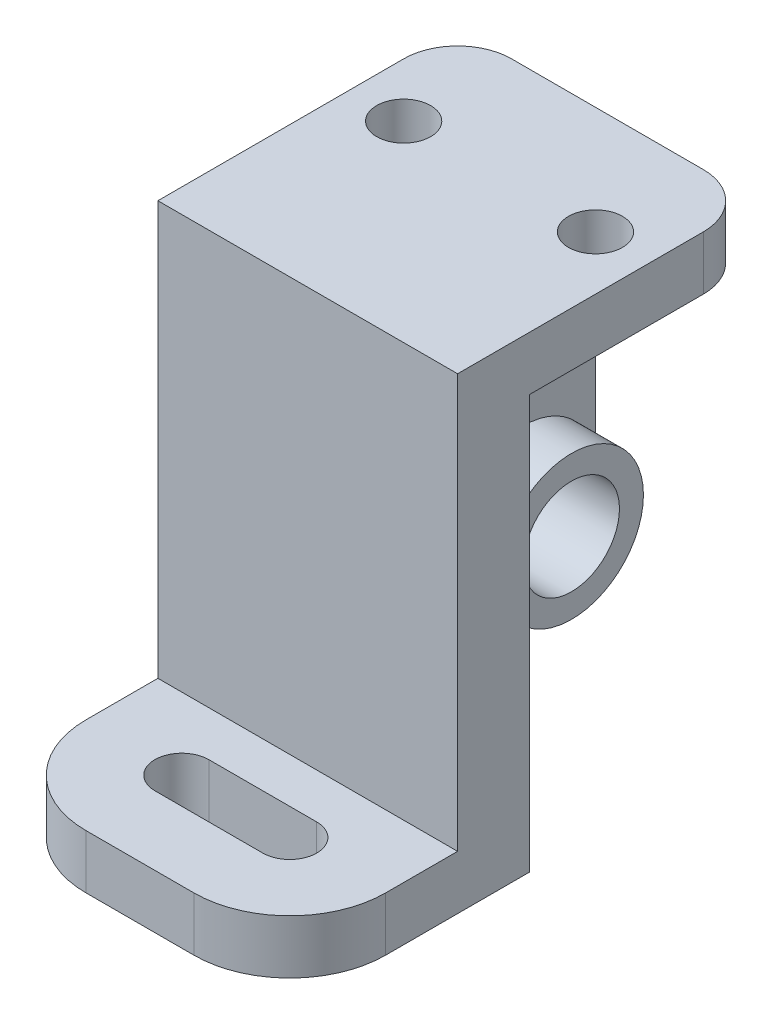
ISO-10303-21;
HEADER;
FILE_DESCRIPTION(('STEP AP214'),'2;1');
FILE_NAME('part.step','',(''),(''),'','','');
FILE_SCHEMA(('AUTOMOTIVE_DESIGN { 1 0 10303 214 1 1 1 1 }'));
ENDSEC;
DATA;
#1=APPLICATION_CONTEXT('core data for automotive mechanical design processes');
#2=APPLICATION_PROTOCOL_DEFINITION('international standard','automotive_design',2000,#1);
#3=PRODUCT_CONTEXT('',#1,'mechanical');
#4=PRODUCT('Part','Part','',(#3));
#5=PRODUCT_RELATED_PRODUCT_CATEGORY('part','',(#4));
#6=PRODUCT_DEFINITION_FORMATION('','',#4);
#7=PRODUCT_DEFINITION_CONTEXT('part definition',#1,'design');
#8=PRODUCT_DEFINITION('design','',#6,#7);
#9=PRODUCT_DEFINITION_SHAPE('','',#8);
#10=(LENGTH_UNIT() NAMED_UNIT(*) SI_UNIT(.MILLI.,.METRE.));
#11=(NAMED_UNIT(*) PLANE_ANGLE_UNIT() SI_UNIT($,.RADIAN.));
#12=(NAMED_UNIT(*) SI_UNIT($,.STERADIAN.) SOLID_ANGLE_UNIT());
#13=UNCERTAINTY_MEASURE_WITH_UNIT(LENGTH_MEASURE(1.E-05),#10,'distance_accuracy_value','');
#14=(GEOMETRIC_REPRESENTATION_CONTEXT(3) GLOBAL_UNCERTAINTY_ASSIGNED_CONTEXT((#13)) GLOBAL_UNIT_ASSIGNED_CONTEXT((#10,
#11,#12)) REPRESENTATION_CONTEXT('',''));
#15=CARTESIAN_POINT('',(0.,0.,0.));
#16=DIRECTION('',(0.,0.,1.));
#17=DIRECTION('',(1.,0.,0.));
#18=AXIS2_PLACEMENT_3D('',#15,#16,#17);
#19=CARTESIAN_POINT('',(-25.,9.,-20.));
#20=DIRECTION('',(0.,0.,1.));
#21=DIRECTION('',(1.,0.,0.));
#22=AXIS2_PLACEMENT_3D('',#19,#20,#21);
#23=PLANE('',#22);
#24=DIRECTION('',(0.,-1.,0.));
#25=VECTOR('',#24,1.);
#26=CARTESIAN_POINT('',(4.,0.,-20.));
#27=LINE('',#26,#25);
#28=CARTESIAN_POINT('',(4.,69.,-20.));
#29=VERTEX_POINT('',#28);
#30=CARTESIAN_POINT('',(4.,0.,-20.));
#31=VERTEX_POINT('',#30);
#32=EDGE_CURVE('E424',#29,#31,#27,.T.);
#33=ORIENTED_EDGE('',*,*,#32,.F.);
#34=DIRECTION('',(-1.,0.,0.));
#35=VECTOR('',#34,1.);
#36=CARTESIAN_POINT('',(0.,69.,-20.));
#37=LINE('',#36,#35);
#38=CARTESIAN_POINT('',(25.,69.,-20.));
#39=VERTEX_POINT('',#38);
#40=EDGE_CURVE('E66',#39,#29,#37,.T.);
#41=ORIENTED_EDGE('',*,*,#40,.F.);
#42=DIRECTION('',(0.,-1.,0.));
#43=VECTOR('',#42,1.);
#44=CARTESIAN_POINT('',(25.,9.,-20.));
#45=LINE('',#44,#43);
#46=CARTESIAN_POINT('',(25.,0.,-20.));
#47=VERTEX_POINT('',#46);
#48=EDGE_CURVE('E341',#39,#47,#45,.T.);
#49=ORIENTED_EDGE('',*,*,#48,.T.);
#50=DIRECTION('',(-1.,0.,0.));
#51=VECTOR('',#50,1.);
#52=CARTESIAN_POINT('',(-25.,0.,-20.));
#53=LINE('',#52,#51);
#54=EDGE_CURVE('E319',#47,#31,#53,.T.);
#55=ORIENTED_EDGE('',*,*,#54,.T.);
#56=EDGE_LOOP('',(#33,#41,#49,#55));
#57=FACE_BOUND('',#56,.T.);
#58=ADVANCED_FACE('F43',(#57),#23,.F.);
#59=CARTESIAN_POINT('',(0.,69.,0.));
#60=DIRECTION('',(0.,1.,0.));
#61=DIRECTION('',(0.,0.,1.));
#62=AXIS2_PLACEMENT_3D('',#59,#60,#61);
#63=PLANE('',#62);
#64=CARTESIAN_POINT('',(16.,69.,-40.));
#65=DIRECTION('',(0.,1.,0.));
#66=DIRECTION('',(0.,0.,1.));
#67=AXIS2_PLACEMENT_3D('',#64,#65,#66);
#68=CIRCLE('',#67,4.5);
#69=CARTESIAN_POINT('',(16.,69.,-35.5));
#70=VERTEX_POINT('',#69);
#71=EDGE_CURVE('E227',#70,#70,#68,.T.);
#72=ORIENTED_EDGE('',*,*,#71,.T.);
#73=EDGE_LOOP('',(#72));
#74=FACE_BOUND('',#73,.T.);
#75=DIRECTION('',(0.,0.,1.));
#76=VECTOR('',#75,1.);
#77=CARTESIAN_POINT('',(4.,69.,-20.));
#78=LINE('',#77,#76);
#79=CARTESIAN_POINT('',(4.,69.,-58.));
#80=VERTEX_POINT('',#79);
#81=EDGE_CURVE('E436',#80,#29,#78,.T.);
#82=ORIENTED_EDGE('',*,*,#81,.F.);
#83=DIRECTION('',(1.,0.,0.));
#84=VECTOR('',#83,1.);
#85=CARTESIAN_POINT('',(0.,69.,-58.));
#86=LINE('',#85,#84);
#87=CARTESIAN_POINT('',(16.,69.,-58.));
#88=VERTEX_POINT('',#87);
#89=EDGE_CURVE('E233',#80,#88,#86,.T.);
#90=ORIENTED_EDGE('',*,*,#89,.T.);
#91=CARTESIAN_POINT('',(16.,69.,-49.));
#92=DIRECTION('',(0.,1.,0.));
#93=DIRECTION('',(0.,0.,1.));
#94=AXIS2_PLACEMENT_3D('',#91,#92,#93);
#95=CIRCLE('',#94,9.);
#96=CARTESIAN_POINT('',(25.,69.,-49.));
#97=VERTEX_POINT('',#96);
#98=EDGE_CURVE('E242',#88,#97,#95,.F.);
#99=ORIENTED_EDGE('',*,*,#98,.T.);
#100=DIRECTION('',(0.,0.,1.));
#101=VECTOR('',#100,1.);
#102=CARTESIAN_POINT('',(25.,69.,0.));
#103=LINE('',#102,#101);
#104=EDGE_CURVE('E241',#97,#39,#103,.T.);
#105=ORIENTED_EDGE('',*,*,#104,.T.);
#106=ORIENTED_EDGE('',*,*,#40,.T.);
#107=EDGE_LOOP('',(#82,#90,#99,#105,#106));
#108=FACE_BOUND('',#107,.T.);
#109=ADVANCED_FACE('F434',(#74,#108),#63,.F.);
#110=CARTESIAN_POINT('',(-4.,69.,-20.));
#111=VERTEX_POINT('',#110);
#112=CARTESIAN_POINT('',(-25.,69.,-20.));
#113=VERTEX_POINT('',#112);
#114=EDGE_CURVE('E237',#111,#113,#37,.T.);
#115=ORIENTED_EDGE('',*,*,#114,.F.);
#116=DIRECTION('',(0.,-1.,0.));
#117=VECTOR('',#116,1.);
#118=CARTESIAN_POINT('',(-4.,0.,-20.));
#119=LINE('',#118,#117);
#120=CARTESIAN_POINT('',(-4.,0.,-20.));
#121=VERTEX_POINT('',#120);
#122=EDGE_CURVE('E59',#111,#121,#119,.T.);
#123=ORIENTED_EDGE('',*,*,#122,.T.);
#124=CARTESIAN_POINT('',(-25.,0.,-20.));
#125=VERTEX_POINT('',#124);
#126=EDGE_CURVE('E339',#121,#125,#53,.T.);
#127=ORIENTED_EDGE('',*,*,#126,.T.);
#128=DIRECTION('',(0.,-1.,0.));
#129=VECTOR('',#128,1.);
#130=CARTESIAN_POINT('',(-25.,9.,-20.));
#131=LINE('',#130,#129);
#132=EDGE_CURVE('E330',#113,#125,#131,.T.);
#133=ORIENTED_EDGE('',*,*,#132,.F.);
#134=EDGE_LOOP('',(#115,#123,#127,#133));
#135=FACE_BOUND('',#134,.T.);
#136=ADVANCED_FACE('F408',(#135),#23,.F.);
#137=CARTESIAN_POINT('',(-9.00000000000001,9.,4.));
#138=DIRECTION('',(0.,1.,0.));
#139=DIRECTION('',(0.,0.,1.));
#140=AXIS2_PLACEMENT_3D('',#137,#138,#139);
#141=PLANE('',#140);
#142=DIRECTION('',(1.,0.,0.));
#143=VECTOR('',#142,1.);
#144=CARTESIAN_POINT('',(-9.00000000000001,9.,8.5));
#145=LINE('',#144,#143);
#146=CARTESIAN_POINT('',(-9.00000000000001,9.,8.5));
#147=VERTEX_POINT('',#146);
#148=CARTESIAN_POINT('',(9.,9.,8.50000000000001));
#149=VERTEX_POINT('',#148);
#150=EDGE_CURVE('E288',#147,#149,#145,.T.);
#151=ORIENTED_EDGE('',*,*,#150,.F.);
#152=CARTESIAN_POINT('',(-9.00000000000001,9.,4.));
#153=DIRECTION('',(0.,1.,0.));
#154=DIRECTION('',(0.,0.,1.));
#155=AXIS2_PLACEMENT_3D('',#152,#153,#154);
#156=CIRCLE('',#155,4.5);
#157=CARTESIAN_POINT('',(-9.00000000000001,9.,-0.499999999999996));
#158=VERTEX_POINT('',#157);
#159=EDGE_CURVE('E282',#158,#147,#156,.T.);
#160=ORIENTED_EDGE('',*,*,#159,.F.);
#161=DIRECTION('',(-1.,0.,0.));
#162=VECTOR('',#161,1.);
#163=CARTESIAN_POINT('',(-9.00000000000001,9.,-0.499999999999996));
#164=LINE('',#163,#162);
#165=CARTESIAN_POINT('',(9.,9.,-0.499999999999994));
#166=VERTEX_POINT('',#165);
#167=EDGE_CURVE('E292',#166,#158,#164,.T.);
#168=ORIENTED_EDGE('',*,*,#167,.F.);
#169=CARTESIAN_POINT('',(9.,9.,4.00000000000001));
#170=DIRECTION('',(0.,1.,0.));
#171=DIRECTION('',(0.,0.,1.));
#172=AXIS2_PLACEMENT_3D('',#169,#170,#171);
#173=CIRCLE('',#172,4.5);
#174=EDGE_CURVE('E287',#149,#166,#173,.T.);
#175=ORIENTED_EDGE('',*,*,#174,.F.);
#176=EDGE_LOOP('',(#151,#160,#168,#175));
#177=FACE_BOUND('',#176,.T.);
#178=DIRECTION('',(0.,0.,-1.));
#179=VECTOR('',#178,1.);
#180=CARTESIAN_POINT('',(25.,9.,-20.));
#181=LINE('',#180,#179);
#182=CARTESIAN_POINT('',(25.,9.,3.99999999999989));
#183=VERTEX_POINT('',#182);
#184=CARTESIAN_POINT('',(25.,9.,-8.));
#185=VERTEX_POINT('',#184);
#186=EDGE_CURVE('E321',#183,#185,#181,.T.);
#187=ORIENTED_EDGE('',*,*,#186,.T.);
#188=DIRECTION('',(-1.,0.,0.));
#189=VECTOR('',#188,1.);
#190=CARTESIAN_POINT('',(25.,9.,-8.));
#191=LINE('',#190,#189);
#192=CARTESIAN_POINT('',(-25.,9.,-8.));
#193=VERTEX_POINT('',#192);
#194=EDGE_CURVE('E269',#185,#193,#191,.T.);
#195=ORIENTED_EDGE('',*,*,#194,.T.);
#196=DIRECTION('',(0.,0.,1.));
#197=VECTOR('',#196,1.);
#198=CARTESIAN_POINT('',(-25.,9.,-20.));
#199=LINE('',#198,#197);
#200=CARTESIAN_POINT('',(-25.,9.,3.99999999999989));
#201=VERTEX_POINT('',#200);
#202=EDGE_CURVE('E314',#193,#201,#199,.T.);
#203=ORIENTED_EDGE('',*,*,#202,.T.);
#204=CARTESIAN_POINT('',(-9.00000000000001,9.,4.));
#205=DIRECTION('',(0.,1.,0.));
#206=DIRECTION('',(0.,0.,1.));
#207=AXIS2_PLACEMENT_3D('',#204,#205,#206);
#208=CIRCLE('',#207,16.);
#209=CARTESIAN_POINT('',(-8.99999999999989,9.,20.));
#210=VERTEX_POINT('',#209);
#211=EDGE_CURVE('E320',#201,#210,#208,.T.);
#212=ORIENTED_EDGE('',*,*,#211,.T.);
#213=DIRECTION('',(1.,0.,0.));
#214=VECTOR('',#213,1.);
#215=CARTESIAN_POINT('',(-8.99999999999989,9.,20.));
#216=LINE('',#215,#214);
#217=CARTESIAN_POINT('',(8.99999999999989,9.,20.));
#218=VERTEX_POINT('',#217);
#219=EDGE_CURVE('E318',#210,#218,#216,.T.);
#220=ORIENTED_EDGE('',*,*,#219,.T.);
#221=CARTESIAN_POINT('',(9.,9.,4.00000000000001));
#222=DIRECTION('',(0.,1.,0.));
#223=DIRECTION('',(0.,0.,1.));
#224=AXIS2_PLACEMENT_3D('',#221,#222,#223);
#225=CIRCLE('',#224,16.);
#226=EDGE_CURVE('E325',#218,#183,#225,.T.);
#227=ORIENTED_EDGE('',*,*,#226,.T.);
#228=EDGE_LOOP('',(#187,#195,#203,#212,#220,#227));
#229=FACE_BOUND('',#228,.T.);
#230=ADVANCED_FACE('F384',(#177,#229),#141,.T.);
#231=CARTESIAN_POINT('',(-9.00000000000001,0.,4.));
#232=DIRECTION('',(0.,1.,0.));
#233=DIRECTION('',(0.,0.,1.));
#234=AXIS2_PLACEMENT_3D('',#231,#232,#233);
#235=PLANE('',#234);
#236=DIRECTION('',(0.,0.,1.));
#237=VECTOR('',#236,1.);
#238=CARTESIAN_POINT('',(-25.,0.,-20.));
#239=LINE('',#238,#237);
#240=CARTESIAN_POINT('',(-25.,0.,3.99999999999989));
#241=VERTEX_POINT('',#240);
#242=EDGE_CURVE('E313',#125,#241,#239,.T.);
#243=ORIENTED_EDGE('',*,*,#242,.F.);
#244=ORIENTED_EDGE('',*,*,#126,.F.);
#245=DIRECTION('',(-1.,0.,0.));
#246=VECTOR('',#245,1.);
#247=CARTESIAN_POINT('',(4.,0.,-20.));
#248=LINE('',#247,#246);
#249=EDGE_CURVE('E416',#31,#121,#248,.T.);
#250=ORIENTED_EDGE('',*,*,#249,.F.);
#251=ORIENTED_EDGE('',*,*,#54,.F.);
#252=DIRECTION('',(0.,0.,-1.));
#253=VECTOR('',#252,1.);
#254=CARTESIAN_POINT('',(25.,0.,-20.));
#255=LINE('',#254,#253);
#256=CARTESIAN_POINT('',(25.,0.,3.99999999999989));
#257=VERTEX_POINT('',#256);
#258=EDGE_CURVE('E337',#257,#47,#255,.T.);
#259=ORIENTED_EDGE('',*,*,#258,.F.);
#260=CARTESIAN_POINT('',(9.,0.,4.00000000000001));
#261=DIRECTION('',(0.,1.,0.));
#262=DIRECTION('',(0.,0.,1.));
#263=AXIS2_PLACEMENT_3D('',#260,#261,#262);
#264=CIRCLE('',#263,16.);
#265=CARTESIAN_POINT('',(8.99999999999989,0.,20.));
#266=VERTEX_POINT('',#265);
#267=EDGE_CURVE('E332',#266,#257,#264,.T.);
#268=ORIENTED_EDGE('',*,*,#267,.F.);
#269=DIRECTION('',(1.,0.,0.));
#270=VECTOR('',#269,1.);
#271=CARTESIAN_POINT('',(-8.99999999999989,0.,20.));
#272=LINE('',#271,#270);
#273=CARTESIAN_POINT('',(-8.99999999999989,0.,20.));
#274=VERTEX_POINT('',#273);
#275=EDGE_CURVE('E335',#274,#266,#272,.T.);
#276=ORIENTED_EDGE('',*,*,#275,.F.);
#277=CARTESIAN_POINT('',(-9.00000000000001,0.,4.));
#278=DIRECTION('',(0.,1.,0.));
#279=DIRECTION('',(0.,0.,1.));
#280=AXIS2_PLACEMENT_3D('',#277,#278,#279);
#281=CIRCLE('',#280,16.);
#282=EDGE_CURVE('E329',#241,#274,#281,.T.);
#283=ORIENTED_EDGE('',*,*,#282,.F.);
#284=EDGE_LOOP('',(#243,#244,#250,#251,#259,#268,#276,#283));
#285=FACE_BOUND('',#284,.T.);
#286=CARTESIAN_POINT('',(-9.00000000000001,0.,4.));
#287=DIRECTION('',(0.,1.,0.));
#288=DIRECTION('',(0.,0.,1.));
#289=AXIS2_PLACEMENT_3D('',#286,#287,#288);
#290=CIRCLE('',#289,4.5);
#291=CARTESIAN_POINT('',(-9.00000000000001,0.,-0.499999999999996));
#292=VERTEX_POINT('',#291);
#293=CARTESIAN_POINT('',(-9.00000000000001,0.,8.5));
#294=VERTEX_POINT('',#293);
#295=EDGE_CURVE('E285',#292,#294,#290,.T.);
#296=ORIENTED_EDGE('',*,*,#295,.T.);
#297=DIRECTION('',(1.,0.,0.));
#298=VECTOR('',#297,1.);
#299=CARTESIAN_POINT('',(-9.00000000000001,0.,8.5));
#300=LINE('',#299,#298);
#301=CARTESIAN_POINT('',(9.,0.,8.50000000000001));
#302=VERTEX_POINT('',#301);
#303=EDGE_CURVE('E300',#294,#302,#300,.T.);
#304=ORIENTED_EDGE('',*,*,#303,.T.);
#305=CARTESIAN_POINT('',(9.,0.,4.00000000000001));
#306=DIRECTION('',(0.,1.,0.));
#307=DIRECTION('',(0.,0.,1.));
#308=AXIS2_PLACEMENT_3D('',#305,#306,#307);
#309=CIRCLE('',#308,4.5);
#310=CARTESIAN_POINT('',(9.,0.,-0.499999999999994));
#311=VERTEX_POINT('',#310);
#312=EDGE_CURVE('E297',#302,#311,#309,.T.);
#313=ORIENTED_EDGE('',*,*,#312,.T.);
#314=DIRECTION('',(-1.,0.,0.));
#315=VECTOR('',#314,1.);
#316=CARTESIAN_POINT('',(-9.00000000000001,0.,-0.499999999999996));
#317=LINE('',#316,#315);
#318=EDGE_CURVE('E290',#311,#292,#317,.T.);
#319=ORIENTED_EDGE('',*,*,#318,.T.);
#320=EDGE_LOOP('',(#296,#304,#313,#319));
#321=FACE_BOUND('',#320,.T.);
#322=ADVANCED_FACE('F370',(#285,#321),#235,.F.);
#323=CARTESIAN_POINT('',(-25.,9.,-20.));
#324=DIRECTION('',(1.,0.,0.));
#325=DIRECTION('',(0.,0.,-1.));
#326=AXIS2_PLACEMENT_3D('',#323,#324,#325);
#327=PLANE('',#326);
#328=ORIENTED_EDGE('',*,*,#242,.T.);
#329=DIRECTION('',(0.,-1.,0.));
#330=VECTOR('',#329,1.);
#331=CARTESIAN_POINT('',(-25.,9.,3.99999999999989));
#332=LINE('',#331,#330);
#333=EDGE_CURVE('E51',#201,#241,#332,.T.);
#334=ORIENTED_EDGE('',*,*,#333,.F.);
#335=ORIENTED_EDGE('',*,*,#202,.F.);
#336=DIRECTION('',(0.,1.,0.));
#337=VECTOR('',#336,1.);
#338=CARTESIAN_POINT('',(-25.,9.,-8.));
#339=LINE('',#338,#337);
#340=CARTESIAN_POINT('',(-25.,78.,-8.));
#341=VERTEX_POINT('',#340);
#342=EDGE_CURVE('E271',#193,#341,#339,.T.);
#343=ORIENTED_EDGE('',*,*,#342,.T.);
#344=DIRECTION('',(0.,0.,-1.));
#345=VECTOR('',#344,1.);
#346=CARTESIAN_POINT('',(-25.,78.,-8.));
#347=LINE('',#346,#345);
#348=CARTESIAN_POINT('',(-25.,78.,-49.));
#349=VERTEX_POINT('',#348);
#350=EDGE_CURVE('E276',#341,#349,#347,.T.);
#351=ORIENTED_EDGE('',*,*,#350,.T.);
#352=DIRECTION('',(0.,1.,0.));
#353=VECTOR('',#352,1.);
#354=CARTESIAN_POINT('',(-25.,69.,-49.));
#355=LINE('',#354,#353);
#356=CARTESIAN_POINT('',(-25.,69.,-49.));
#357=VERTEX_POINT('',#356);
#358=EDGE_CURVE('E263',#357,#349,#355,.T.);
#359=ORIENTED_EDGE('',*,*,#358,.F.);
#360=DIRECTION('',(0.,0.,-1.));
#361=VECTOR('',#360,1.);
#362=CARTESIAN_POINT('',(-25.,69.,0.));
#363=LINE('',#362,#361);
#364=EDGE_CURVE('E240',#113,#357,#363,.T.);
#365=ORIENTED_EDGE('',*,*,#364,.F.);
#366=ORIENTED_EDGE('',*,*,#132,.T.);
#367=EDGE_LOOP('',(#328,#334,#335,#343,#351,#359,#365,#366));
#368=FACE_BOUND('',#367,.T.);
#369=ADVANCED_FACE('F44',(#368),#327,.F.);
#370=CARTESIAN_POINT('',(-9.00000000000001,9.,4.));
#371=DIRECTION('',(0.,-1.,0.));
#372=DIRECTION('',(0.,0.,-1.));
#373=AXIS2_PLACEMENT_3D('',#370,#371,#372);
#374=CYLINDRICAL_SURFACE('',#373,16.);
#375=ORIENTED_EDGE('',*,*,#282,.T.);
#376=DIRECTION('',(0.,-1.,0.));
#377=VECTOR('',#376,1.);
#378=CARTESIAN_POINT('',(-8.99999999999989,9.,20.));
#379=LINE('',#378,#377);
#380=EDGE_CURVE('E355',#210,#274,#379,.T.);
#381=ORIENTED_EDGE('',*,*,#380,.F.);
#382=ORIENTED_EDGE('',*,*,#211,.F.);
#383=ORIENTED_EDGE('',*,*,#333,.T.);
#384=EDGE_LOOP('',(#375,#381,#382,#383));
#385=FACE_BOUND('',#384,.T.);
#386=ADVANCED_FACE('F356',(#385),#374,.T.);
#387=CARTESIAN_POINT('',(-8.99999999999989,9.,20.));
#388=DIRECTION('',(0.,0.,-1.));
#389=DIRECTION('',(-1.,0.,0.));
#390=AXIS2_PLACEMENT_3D('',#387,#388,#389);
#391=PLANE('',#390);
#392=ORIENTED_EDGE('',*,*,#275,.T.);
#393=DIRECTION('',(0.,-1.,0.));
#394=VECTOR('',#393,1.);
#395=CARTESIAN_POINT('',(8.99999999999989,9.,20.));
#396=LINE('',#395,#394);
#397=EDGE_CURVE('E347',#218,#266,#396,.T.);
#398=ORIENTED_EDGE('',*,*,#397,.F.);
#399=ORIENTED_EDGE('',*,*,#219,.F.);
#400=ORIENTED_EDGE('',*,*,#380,.T.);
#401=EDGE_LOOP('',(#392,#398,#399,#400));
#402=FACE_BOUND('',#401,.T.);
#403=ADVANCED_FACE('F374',(#402),#391,.F.);
#404=CARTESIAN_POINT('',(9.,9.,4.00000000000001));
#405=DIRECTION('',(0.,-1.,0.));
#406=DIRECTION('',(0.,0.,-1.));
#407=AXIS2_PLACEMENT_3D('',#404,#405,#406);
#408=CYLINDRICAL_SURFACE('',#407,16.);
#409=ORIENTED_EDGE('',*,*,#267,.T.);
#410=DIRECTION('',(0.,-1.,0.));
#411=VECTOR('',#410,1.);
#412=CARTESIAN_POINT('',(25.,9.,3.99999999999989));
#413=LINE('',#412,#411);
#414=EDGE_CURVE('E346',#183,#257,#413,.T.);
#415=ORIENTED_EDGE('',*,*,#414,.F.);
#416=ORIENTED_EDGE('',*,*,#226,.F.);
#417=ORIENTED_EDGE('',*,*,#397,.T.);
#418=EDGE_LOOP('',(#409,#415,#416,#417));
#419=FACE_BOUND('',#418,.T.);
#420=ADVANCED_FACE('F378',(#419),#408,.T.);
#421=CARTESIAN_POINT('',(25.,9.,-20.));
#422=DIRECTION('',(-1.,0.,0.));
#423=DIRECTION('',(0.,0.,1.));
#424=AXIS2_PLACEMENT_3D('',#421,#422,#423);
#425=PLANE('',#424);
#426=ORIENTED_EDGE('',*,*,#258,.T.);
#427=ORIENTED_EDGE('',*,*,#48,.F.);
#428=ORIENTED_EDGE('',*,*,#104,.F.);
#429=DIRECTION('',(0.,1.,0.));
#430=VECTOR('',#429,1.);
#431=CARTESIAN_POINT('',(25.,69.,-49.));
#432=LINE('',#431,#430);
#433=CARTESIAN_POINT('',(25.,78.,-49.));
#434=VERTEX_POINT('',#433);
#435=EDGE_CURVE('E258',#97,#434,#432,.T.);
#436=ORIENTED_EDGE('',*,*,#435,.T.);
#437=DIRECTION('',(0.,0.,-1.));
#438=VECTOR('',#437,1.);
#439=CARTESIAN_POINT('',(25.,78.,-8.));
#440=LINE('',#439,#438);
#441=CARTESIAN_POINT('',(25.,78.,-8.));
#442=VERTEX_POINT('',#441);
#443=EDGE_CURVE('E278',#442,#434,#440,.T.);
#444=ORIENTED_EDGE('',*,*,#443,.F.);
#445=DIRECTION('',(0.,-1.,0.));
#446=VECTOR('',#445,1.);
#447=CARTESIAN_POINT('',(25.,9.,-8.));
#448=LINE('',#447,#446);
#449=EDGE_CURVE('E256',#442,#185,#448,.T.);
#450=ORIENTED_EDGE('',*,*,#449,.T.);
#451=ORIENTED_EDGE('',*,*,#186,.F.);
#452=ORIENTED_EDGE('',*,*,#414,.T.);
#453=EDGE_LOOP('',(#426,#427,#428,#436,#444,#450,#451,#452));
#454=FACE_BOUND('',#453,.T.);
#455=ADVANCED_FACE('F426',(#454),#425,.F.);
#456=CARTESIAN_POINT('',(-9.00000000000001,9.,4.));
#457=DIRECTION('',(0.,-1.,0.));
#458=DIRECTION('',(0.,0.,-1.));
#459=AXIS2_PLACEMENT_3D('',#456,#457,#458);
#460=CYLINDRICAL_SURFACE('',#459,4.5);
#461=ORIENTED_EDGE('',*,*,#295,.F.);
#462=DIRECTION('',(0.,-1.,0.));
#463=VECTOR('',#462,1.);
#464=CARTESIAN_POINT('',(-9.00000000000001,9.,-0.499999999999996));
#465=LINE('',#464,#463);
#466=EDGE_CURVE('E295',#158,#292,#465,.T.);
#467=ORIENTED_EDGE('',*,*,#466,.F.);
#468=ORIENTED_EDGE('',*,*,#159,.T.);
#469=DIRECTION('',(0.,-1.,0.));
#470=VECTOR('',#469,1.);
#471=CARTESIAN_POINT('',(-9.00000000000001,9.,8.5));
#472=LINE('',#471,#470);
#473=EDGE_CURVE('E311',#147,#294,#472,.T.);
#474=ORIENTED_EDGE('',*,*,#473,.T.);
#475=EDGE_LOOP('',(#461,#467,#468,#474));
#476=FACE_BOUND('',#475,.T.);
#477=ADVANCED_FACE('F499',(#476),#460,.F.);
#478=CARTESIAN_POINT('',(-9.00000000000001,9.,8.5));
#479=DIRECTION('',(0.,0.,-1.));
#480=DIRECTION('',(-1.,0.,0.));
#481=AXIS2_PLACEMENT_3D('',#478,#479,#480);
#482=PLANE('',#481);
#483=ORIENTED_EDGE('',*,*,#303,.F.);
#484=ORIENTED_EDGE('',*,*,#473,.F.);
#485=ORIENTED_EDGE('',*,*,#150,.T.);
#486=DIRECTION('',(0.,-1.,0.));
#487=VECTOR('',#486,1.);
#488=CARTESIAN_POINT('',(9.,9.,8.50000000000001));
#489=LINE('',#488,#487);
#490=EDGE_CURVE('E307',#149,#302,#489,.T.);
#491=ORIENTED_EDGE('',*,*,#490,.T.);
#492=EDGE_LOOP('',(#483,#484,#485,#491));
#493=FACE_BOUND('',#492,.T.);
#494=ADVANCED_FACE('F503',(#493),#482,.T.);
#495=CARTESIAN_POINT('',(9.,9.,4.00000000000001));
#496=DIRECTION('',(0.,-1.,0.));
#497=DIRECTION('',(0.,0.,-1.));
#498=AXIS2_PLACEMENT_3D('',#495,#496,#497);
#499=CYLINDRICAL_SURFACE('',#498,4.5);
#500=ORIENTED_EDGE('',*,*,#312,.F.);
#501=ORIENTED_EDGE('',*,*,#490,.F.);
#502=ORIENTED_EDGE('',*,*,#174,.T.);
#503=DIRECTION('',(0.,-1.,0.));
#504=VECTOR('',#503,1.);
#505=CARTESIAN_POINT('',(9.,9.,-0.499999999999994));
#506=LINE('',#505,#504);
#507=EDGE_CURVE('E310',#166,#311,#506,.T.);
#508=ORIENTED_EDGE('',*,*,#507,.T.);
#509=EDGE_LOOP('',(#500,#501,#502,#508));
#510=FACE_BOUND('',#509,.T.);
#511=ADVANCED_FACE('F510',(#510),#499,.F.);
#512=CARTESIAN_POINT('',(-9.00000000000001,9.,-0.499999999999996));
#513=DIRECTION('',(0.,0.,1.));
#514=DIRECTION('',(1.,0.,0.));
#515=AXIS2_PLACEMENT_3D('',#512,#513,#514);
#516=PLANE('',#515);
#517=ORIENTED_EDGE('',*,*,#318,.F.);
#518=ORIENTED_EDGE('',*,*,#507,.F.);
#519=ORIENTED_EDGE('',*,*,#167,.T.);
#520=ORIENTED_EDGE('',*,*,#466,.T.);
#521=EDGE_LOOP('',(#517,#518,#519,#520));
#522=FACE_BOUND('',#521,.T.);
#523=ADVANCED_FACE('F512',(#522),#516,.T.);
#524=CARTESIAN_POINT('',(25.,78.,-8.));
#525=DIRECTION('',(0.,1.,0.));
#526=DIRECTION('',(0.,0.,1.));
#527=AXIS2_PLACEMENT_3D('',#524,#525,#526);
#528=PLANE('',#527);
#529=ORIENTED_EDGE('',*,*,#443,.T.);
#530=CARTESIAN_POINT('',(16.,78.,-49.));
#531=DIRECTION('',(0.,1.,0.));
#532=DIRECTION('',(0.,0.,1.));
#533=AXIS2_PLACEMENT_3D('',#530,#531,#532);
#534=CIRCLE('',#533,9.);
#535=CARTESIAN_POINT('',(16.,78.,-58.));
#536=VERTEX_POINT('',#535);
#537=EDGE_CURVE('E226',#536,#434,#534,.F.);
#538=ORIENTED_EDGE('',*,*,#537,.F.);
#539=DIRECTION('',(1.,0.,0.));
#540=VECTOR('',#539,1.);
#541=CARTESIAN_POINT('',(0.,78.,-58.));
#542=LINE('',#541,#540);
#543=CARTESIAN_POINT('',(-16.,78.,-58.));
#544=VERTEX_POINT('',#543);
#545=EDGE_CURVE('E248',#544,#536,#542,.T.);
#546=ORIENTED_EDGE('',*,*,#545,.F.);
#547=CARTESIAN_POINT('',(-16.,78.,-49.));
#548=DIRECTION('',(0.,1.,0.));
#549=DIRECTION('',(0.,0.,1.));
#550=AXIS2_PLACEMENT_3D('',#547,#548,#549);
#551=CIRCLE('',#550,9.);
#552=EDGE_CURVE('E255',#349,#544,#551,.F.);
#553=ORIENTED_EDGE('',*,*,#552,.F.);
#554=ORIENTED_EDGE('',*,*,#350,.F.);
#555=DIRECTION('',(1.,0.,0.));
#556=VECTOR('',#555,1.);
#557=CARTESIAN_POINT('',(25.,78.,-8.));
#558=LINE('',#557,#556);
#559=EDGE_CURVE('E277',#341,#442,#558,.T.);
#560=ORIENTED_EDGE('',*,*,#559,.T.);
#561=EDGE_LOOP('',(#529,#538,#546,#553,#554,#560));
#562=FACE_BOUND('',#561,.T.);
#563=CARTESIAN_POINT('',(-16.,78.,-40.));
#564=DIRECTION('',(0.,1.,0.));
#565=DIRECTION('',(0.,0.,1.));
#566=AXIS2_PLACEMENT_3D('',#563,#564,#565);
#567=CIRCLE('',#566,4.5);
#568=CARTESIAN_POINT('',(-16.,78.,-35.5));
#569=VERTEX_POINT('',#568);
#570=EDGE_CURVE('E211',#569,#569,#567,.T.);
#571=ORIENTED_EDGE('',*,*,#570,.F.);
#572=EDGE_LOOP('',(#571));
#573=FACE_BOUND('',#572,.T.);
#574=CARTESIAN_POINT('',(16.,78.,-40.));
#575=DIRECTION('',(0.,1.,0.));
#576=DIRECTION('',(0.,0.,1.));
#577=AXIS2_PLACEMENT_3D('',#574,#575,#576);
#578=CIRCLE('',#577,4.5);
#579=CARTESIAN_POINT('',(16.,78.,-35.5));
#580=VERTEX_POINT('',#579);
#581=EDGE_CURVE('E218',#580,#580,#578,.T.);
#582=ORIENTED_EDGE('',*,*,#581,.F.);
#583=EDGE_LOOP('',(#582));
#584=FACE_BOUND('',#583,.T.);
#585=ADVANCED_FACE('F388',(#562,#573,#584),#528,.T.);
#586=CARTESIAN_POINT('',(0.,0.,-8.));
#587=DIRECTION('',(0.,0.,1.));
#588=DIRECTION('',(1.,0.,0.));
#589=AXIS2_PLACEMENT_3D('',#586,#587,#588);
#590=PLANE('',#589);
#591=ORIENTED_EDGE('',*,*,#449,.F.);
#592=ORIENTED_EDGE('',*,*,#559,.F.);
#593=ORIENTED_EDGE('',*,*,#342,.F.);
#594=ORIENTED_EDGE('',*,*,#194,.F.);
#595=EDGE_LOOP('',(#591,#592,#593,#594));
#596=FACE_BOUND('',#595,.T.);
#597=ADVANCED_FACE('F389',(#596),#590,.T.);
#598=CARTESIAN_POINT('',(0.,69.,-58.));
#599=DIRECTION('',(0.,0.,1.));
#600=DIRECTION('',(1.,0.,0.));
#601=AXIS2_PLACEMENT_3D('',#598,#599,#600);
#602=PLANE('',#601);
#603=ORIENTED_EDGE('',*,*,#545,.T.);
#604=DIRECTION('',(0.,1.,0.));
#605=VECTOR('',#604,1.);
#606=CARTESIAN_POINT('',(16.,69.,-58.));
#607=LINE('',#606,#605);
#608=EDGE_CURVE('E257',#88,#536,#607,.T.);
#609=ORIENTED_EDGE('',*,*,#608,.F.);
#610=ORIENTED_EDGE('',*,*,#89,.F.);
#611=DIRECTION('',(-1.,0.,0.));
#612=VECTOR('',#611,1.);
#613=CARTESIAN_POINT('',(4.,69.,-58.));
#614=LINE('',#613,#612);
#615=CARTESIAN_POINT('',(-4.,69.,-58.));
#616=VERTEX_POINT('',#615);
#617=EDGE_CURVE('E219',#80,#616,#614,.T.);
#618=ORIENTED_EDGE('',*,*,#617,.T.);
#619=CARTESIAN_POINT('',(-16.,69.,-58.));
#620=VERTEX_POINT('',#619);
#621=EDGE_CURVE('E235',#620,#616,#86,.T.);
#622=ORIENTED_EDGE('',*,*,#621,.F.);
#623=DIRECTION('',(0.,1.,0.));
#624=VECTOR('',#623,1.);
#625=CARTESIAN_POINT('',(-16.,69.,-58.));
#626=LINE('',#625,#624);
#627=EDGE_CURVE('E244',#620,#544,#626,.T.);
#628=ORIENTED_EDGE('',*,*,#627,.T.);
#629=EDGE_LOOP('',(#603,#609,#610,#618,#622,#628));
#630=FACE_BOUND('',#629,.T.);
#631=ADVANCED_FACE('F399',(#630),#602,.F.);
#632=CARTESIAN_POINT('',(16.,69.,-49.));
#633=DIRECTION('',(0.,1.,0.));
#634=DIRECTION('',(0.,0.,1.));
#635=AXIS2_PLACEMENT_3D('',#632,#633,#634);
#636=CYLINDRICAL_SURFACE('',#635,9.);
#637=ORIENTED_EDGE('',*,*,#537,.T.);
#638=ORIENTED_EDGE('',*,*,#435,.F.);
#639=ORIENTED_EDGE('',*,*,#98,.F.);
#640=ORIENTED_EDGE('',*,*,#608,.T.);
#641=EDGE_LOOP('',(#637,#638,#639,#640));
#642=FACE_BOUND('',#641,.T.);
#643=ADVANCED_FACE('F435',(#642),#636,.T.);
#644=CARTESIAN_POINT('',(16.,69.,-40.));
#645=DIRECTION('',(0.,1.,0.));
#646=DIRECTION('',(0.,0.,1.));
#647=AXIS2_PLACEMENT_3D('',#644,#645,#646);
#648=CYLINDRICAL_SURFACE('',#647,4.5);
#649=ORIENTED_EDGE('',*,*,#71,.F.);
#650=EDGE_LOOP('',(#649));
#651=FACE_BOUND('',#650,.T.);
#652=ORIENTED_EDGE('',*,*,#581,.T.);
#653=EDGE_LOOP('',(#652));
#654=FACE_BOUND('',#653,.T.);
#655=ADVANCED_FACE('F521',(#651,#654),#648,.F.);
#656=CARTESIAN_POINT('',(-16.,69.,-40.));
#657=DIRECTION('',(0.,1.,0.));
#658=DIRECTION('',(0.,0.,1.));
#659=AXIS2_PLACEMENT_3D('',#656,#657,#658);
#660=CYLINDRICAL_SURFACE('',#659,4.5);
#661=CARTESIAN_POINT('',(-16.,69.,-40.));
#662=DIRECTION('',(0.,1.,0.));
#663=DIRECTION('',(0.,0.,1.));
#664=AXIS2_PLACEMENT_3D('',#661,#662,#663);
#665=CIRCLE('',#664,4.5);
#666=CARTESIAN_POINT('',(-16.,69.,-35.5));
#667=VERTEX_POINT('',#666);
#668=EDGE_CURVE('E222',#667,#667,#665,.T.);
#669=ORIENTED_EDGE('',*,*,#668,.F.);
#670=EDGE_LOOP('',(#669));
#671=FACE_BOUND('',#670,.T.);
#672=ORIENTED_EDGE('',*,*,#570,.T.);
#673=EDGE_LOOP('',(#672));
#674=FACE_BOUND('',#673,.T.);
#675=ADVANCED_FACE('F519',(#671,#674),#660,.F.);
#676=CARTESIAN_POINT('',(-16.,69.,-49.));
#677=DIRECTION('',(0.,1.,0.));
#678=DIRECTION('',(0.,0.,1.));
#679=AXIS2_PLACEMENT_3D('',#676,#677,#678);
#680=CYLINDRICAL_SURFACE('',#679,9.);
#681=ORIENTED_EDGE('',*,*,#552,.T.);
#682=ORIENTED_EDGE('',*,*,#627,.F.);
#683=CARTESIAN_POINT('',(-16.,69.,-49.));
#684=DIRECTION('',(0.,1.,0.));
#685=DIRECTION('',(0.,0.,1.));
#686=AXIS2_PLACEMENT_3D('',#683,#684,#685);
#687=CIRCLE('',#686,9.);
#688=EDGE_CURVE('E232',#357,#620,#687,.F.);
#689=ORIENTED_EDGE('',*,*,#688,.F.);
#690=ORIENTED_EDGE('',*,*,#358,.T.);
#691=EDGE_LOOP('',(#681,#682,#689,#690));
#692=FACE_BOUND('',#691,.T.);
#693=ADVANCED_FACE('F398',(#692),#680,.T.);
#694=ORIENTED_EDGE('',*,*,#668,.T.);
#695=EDGE_LOOP('',(#694));
#696=FACE_BOUND('',#695,.T.);
#697=ORIENTED_EDGE('',*,*,#621,.T.);
#698=DIRECTION('',(0.,0.,1.));
#699=VECTOR('',#698,1.);
#700=CARTESIAN_POINT('',(-4.,69.,-20.));
#701=LINE('',#700,#699);
#702=EDGE_CURVE('E410',#616,#111,#701,.T.);
#703=ORIENTED_EDGE('',*,*,#702,.T.);
#704=ORIENTED_EDGE('',*,*,#114,.T.);
#705=ORIENTED_EDGE('',*,*,#364,.T.);
#706=ORIENTED_EDGE('',*,*,#688,.T.);
#707=EDGE_LOOP('',(#697,#703,#704,#705,#706));
#708=FACE_BOUND('',#707,.T.);
#709=ADVANCED_FACE('F407',(#696,#708),#63,.F.);
#710=CARTESIAN_POINT('',(4.,32.,-40.));
#711=DIRECTION('',(-1.,0.,0.));
#712=DIRECTION('',(0.,0.,1.));
#713=AXIS2_PLACEMENT_3D('',#710,#711,#712);
#714=CYLINDRICAL_SURFACE('',#713,12.);
#715=DIRECTION('',(-1.,0.,0.));
#716=VECTOR('',#715,1.);
#717=CARTESIAN_POINT('',(4.,21.7780089207025,-46.2857695133342));
#718=LINE('',#717,#716);
#719=CARTESIAN_POINT('',(4.,21.7780089207025,-46.2857695133342));
#720=VERTEX_POINT('',#719);
#721=CARTESIAN_POINT('',(-4.,21.7780089207025,-46.2857695133342));
#722=VERTEX_POINT('',#721);
#723=EDGE_CURVE('E199',#720,#722,#718,.T.);
#724=ORIENTED_EDGE('',*,*,#723,.T.);
#725=CARTESIAN_POINT('',(-4.,32.,-40.));
#726=DIRECTION('',(-1.,0.,0.));
#727=DIRECTION('',(0.,0.,1.));
#728=AXIS2_PLACEMENT_3D('',#725,#726,#727);
#729=CIRCLE('',#728,12.);
#730=CARTESIAN_POINT('',(-4.,32.,-52.));
#731=VERTEX_POINT('',#730);
#732=EDGE_CURVE('E11',#731,#722,#729,.F.);
#733=ORIENTED_EDGE('',*,*,#732,.F.);
#734=DIRECTION('',(-1.,0.,0.));
#735=VECTOR('',#734,1.);
#736=CARTESIAN_POINT('',(4.,32.,-52.));
#737=LINE('',#736,#735);
#738=CARTESIAN_POINT('',(4.,32.,-52.));
#739=VERTEX_POINT('',#738);
#740=EDGE_CURVE('E197',#739,#731,#737,.T.);
#741=ORIENTED_EDGE('',*,*,#740,.F.);
#742=CARTESIAN_POINT('',(4.,32.,-40.));
#743=DIRECTION('',(-1.,0.,0.));
#744=DIRECTION('',(0.,0.,1.));
#745=AXIS2_PLACEMENT_3D('',#742,#743,#744);
#746=CIRCLE('',#745,12.);
#747=EDGE_CURVE('E209',#739,#720,#746,.F.);
#748=ORIENTED_EDGE('',*,*,#747,.T.);
#749=EDGE_LOOP('',(#724,#733,#741,#748));
#750=FACE_BOUND('',#749,.T.);
#751=CARTESIAN_POINT('',(-12.,32.,-40.));
#752=DIRECTION('',(1.,0.,0.));
#753=DIRECTION('',(0.,0.,-1.));
#754=AXIS2_PLACEMENT_3D('',#751,#752,#753);
#755=CIRCLE('',#754,12.);
#756=CARTESIAN_POINT('',(-12.,32.,-52.));
#757=VERTEX_POINT('',#756);
#758=EDGE_CURVE('E452',#757,#757,#755,.T.);
#759=ORIENTED_EDGE('',*,*,#758,.T.);
#760=EDGE_LOOP('',(#759));
#761=FACE_BOUND('',#760,.T.);
#762=CARTESIAN_POINT('',(12.,32.,-40.));
#763=DIRECTION('',(1.,0.,0.));
#764=DIRECTION('',(0.,0.,-1.));
#765=AXIS2_PLACEMENT_3D('',#762,#763,#764);
#766=CIRCLE('',#765,12.);
#767=CARTESIAN_POINT('',(12.,32.,-52.));
#768=VERTEX_POINT('',#767);
#769=EDGE_CURVE('E448',#768,#768,#766,.T.);
#770=ORIENTED_EDGE('',*,*,#769,.F.);
#771=EDGE_LOOP('',(#770));
#772=FACE_BOUND('',#771,.T.);
#773=ADVANCED_FACE('F193',(#750,#761,#772),#714,.T.);
#774=CARTESIAN_POINT('',(4.,32.,-52.));
#775=DIRECTION('',(0.,0.,1.));
#776=DIRECTION('',(1.,0.,0.));
#777=AXIS2_PLACEMENT_3D('',#774,#775,#776);
#778=PLANE('',#777);
#779=DIRECTION('',(0.,1.,0.));
#780=VECTOR('',#779,1.);
#781=CARTESIAN_POINT('',(-4.,32.,-52.));
#782=LINE('',#781,#780);
#783=CARTESIAN_POINT('',(-4.,61.4445908841296,-52.));
#784=VERTEX_POINT('',#783);
#785=EDGE_CURVE('E201',#731,#784,#782,.T.);
#786=ORIENTED_EDGE('',*,*,#785,.T.);
#787=DIRECTION('',(-1.,0.,0.));
#788=VECTOR('',#787,1.);
#789=CARTESIAN_POINT('',(4.,61.4445908841296,-52.));
#790=LINE('',#789,#788);
#791=CARTESIAN_POINT('',(4.,61.4445908841296,-52.));
#792=VERTEX_POINT('',#791);
#793=EDGE_CURVE('E213',#792,#784,#790,.T.);
#794=ORIENTED_EDGE('',*,*,#793,.F.);
#795=DIRECTION('',(0.,1.,0.));
#796=VECTOR('',#795,1.);
#797=CARTESIAN_POINT('',(4.,32.,-52.));
#798=LINE('',#797,#796);
#799=EDGE_CURVE('E214',#739,#792,#798,.T.);
#800=ORIENTED_EDGE('',*,*,#799,.F.);
#801=ORIENTED_EDGE('',*,*,#740,.T.);
#802=EDGE_LOOP('',(#786,#794,#800,#801));
#803=FACE_BOUND('',#802,.T.);
#804=ADVANCED_FACE('F215',(#803),#778,.F.);
#805=CARTESIAN_POINT('',(4.,55.7350867836948,-66.9466237969355));
#806=DIRECTION('',(-1.,0.,0.));
#807=DIRECTION('',(0.,0.,1.));
#808=AXIS2_PLACEMENT_3D('',#805,#806,#807);
#809=CYLINDRICAL_SURFACE('',#808,16.);
#810=CARTESIAN_POINT('',(-4.,55.7350867836948,-66.9466237969355));
#811=DIRECTION('',(-1.,0.,0.));
#812=DIRECTION('',(0.,0.,1.));
#813=AXIS2_PLACEMENT_3D('',#810,#811,#812);
#814=CIRCLE('',#813,16.);
#815=EDGE_CURVE('E204',#784,#616,#814,.T.);
#816=ORIENTED_EDGE('',*,*,#815,.T.);
#817=ORIENTED_EDGE('',*,*,#617,.F.);
#818=CARTESIAN_POINT('',(4.,55.7350867836948,-66.9466237969355));
#819=DIRECTION('',(-1.,0.,0.));
#820=DIRECTION('',(0.,0.,1.));
#821=AXIS2_PLACEMENT_3D('',#818,#819,#820);
#822=CIRCLE('',#821,16.);
#823=EDGE_CURVE('E438',#792,#80,#822,.T.);
#824=ORIENTED_EDGE('',*,*,#823,.F.);
#825=ORIENTED_EDGE('',*,*,#793,.T.);
#826=EDGE_LOOP('',(#816,#817,#824,#825));
#827=FACE_BOUND('',#826,.T.);
#828=ADVANCED_FACE('F444',(#827),#809,.F.);
#829=CARTESIAN_POINT('',(4.,0.,-20.));
#830=DIRECTION('',(0.,0.770045000830657,0.637989574127754));
#831=DIRECTION('',(0.,-0.637989574127754,0.770045000830657));
#832=AXIS2_PLACEMENT_3D('',#829,#830,#831);
#833=PLANE('',#832);
#834=DIRECTION('',(0.,0.637989574127754,-0.770045000830657));
#835=VECTOR('',#834,1.);
#836=CARTESIAN_POINT('',(-4.,0.,-20.));
#837=LINE('',#836,#835);
#838=EDGE_CURVE('E411',#121,#722,#837,.T.);
#839=ORIENTED_EDGE('',*,*,#838,.T.);
#840=ORIENTED_EDGE('',*,*,#723,.F.);
#841=DIRECTION('',(0.,0.637989574127754,-0.770045000830657));
#842=VECTOR('',#841,1.);
#843=CARTESIAN_POINT('',(4.,0.,-20.));
#844=LINE('',#843,#842);
#845=EDGE_CURVE('E417',#31,#720,#844,.T.);
#846=ORIENTED_EDGE('',*,*,#845,.F.);
#847=ORIENTED_EDGE('',*,*,#249,.T.);
#848=EDGE_LOOP('',(#839,#840,#846,#847));
#849=FACE_BOUND('',#848,.T.);
#850=ADVANCED_FACE('F422',(#849),#833,.F.);
#851=CARTESIAN_POINT('',(4.,32.,-40.));
#852=DIRECTION('',(-1.,0.,0.));
#853=DIRECTION('',(0.,0.,1.));
#854=AXIS2_PLACEMENT_3D('',#851,#852,#853);
#855=PLANE('',#854);
#856=ORIENTED_EDGE('',*,*,#747,.F.);
#857=ORIENTED_EDGE('',*,*,#799,.T.);
#858=ORIENTED_EDGE('',*,*,#823,.T.);
#859=ORIENTED_EDGE('',*,*,#81,.T.);
#860=ORIENTED_EDGE('',*,*,#32,.T.);
#861=ORIENTED_EDGE('',*,*,#845,.T.);
#862=EDGE_LOOP('',(#856,#857,#858,#859,#860,#861));
#863=FACE_BOUND('',#862,.T.);
#864=ADVANCED_FACE('F450',(#863),#855,.F.);
#865=CARTESIAN_POINT('',(-4.,32.,-40.));
#866=DIRECTION('',(-1.,0.,0.));
#867=DIRECTION('',(0.,0.,1.));
#868=AXIS2_PLACEMENT_3D('',#865,#866,#867);
#869=PLANE('',#868);
#870=ORIENTED_EDGE('',*,*,#785,.F.);
#871=ORIENTED_EDGE('',*,*,#732,.T.);
#872=ORIENTED_EDGE('',*,*,#838,.F.);
#873=ORIENTED_EDGE('',*,*,#122,.F.);
#874=ORIENTED_EDGE('',*,*,#702,.F.);
#875=ORIENTED_EDGE('',*,*,#815,.F.);
#876=EDGE_LOOP('',(#870,#871,#872,#873,#874,#875));
#877=FACE_BOUND('',#876,.T.);
#878=ADVANCED_FACE('F202',(#877),#869,.T.);
#879=CARTESIAN_POINT('',(-12.,32.,-40.));
#880=DIRECTION('',(1.,0.,0.));
#881=DIRECTION('',(0.,0.,-1.));
#882=AXIS2_PLACEMENT_3D('',#879,#880,#881);
#883=PLANE('',#882);
#884=ORIENTED_EDGE('',*,*,#758,.F.);
#885=EDGE_LOOP('',(#884));
#886=FACE_BOUND('',#885,.T.);
#887=CARTESIAN_POINT('',(-12.,32.,-40.));
#888=DIRECTION('',(1.,0.,0.));
#889=DIRECTION('',(0.,0.,-1.));
#890=AXIS2_PLACEMENT_3D('',#887,#888,#889);
#891=CIRCLE('',#890,8.);
#892=CARTESIAN_POINT('',(-12.,32.,-48.));
#893=VERTEX_POINT('',#892);
#894=EDGE_CURVE('E460',#893,#893,#891,.T.);
#895=ORIENTED_EDGE('',*,*,#894,.T.);
#896=EDGE_LOOP('',(#895));
#897=FACE_BOUND('',#896,.T.);
#898=ADVANCED_FACE('F471',(#886,#897),#883,.F.);
#899=CARTESIAN_POINT('',(12.,32.,-40.));
#900=DIRECTION('',(-1.,0.,0.));
#901=DIRECTION('',(0.,0.,1.));
#902=AXIS2_PLACEMENT_3D('',#899,#900,#901);
#903=CYLINDRICAL_SURFACE('',#902,8.);
#904=CARTESIAN_POINT('',(12.,32.,-40.));
#905=DIRECTION('',(1.,0.,0.));
#906=DIRECTION('',(0.,0.,-1.));
#907=AXIS2_PLACEMENT_3D('',#904,#905,#906);
#908=CIRCLE('',#907,8.);
#909=CARTESIAN_POINT('',(12.,32.,-48.));
#910=VERTEX_POINT('',#909);
#911=EDGE_CURVE('E451',#910,#910,#908,.T.);
#912=ORIENTED_EDGE('',*,*,#911,.T.);
#913=EDGE_LOOP('',(#912));
#914=FACE_BOUND('',#913,.T.);
#915=ORIENTED_EDGE('',*,*,#894,.F.);
#916=EDGE_LOOP('',(#915));
#917=FACE_BOUND('',#916,.T.);
#918=ADVANCED_FACE('F461',(#914,#917),#903,.F.);
#919=CARTESIAN_POINT('',(12.,32.,-40.));
#920=DIRECTION('',(1.,0.,0.));
#921=DIRECTION('',(0.,0.,-1.));
#922=AXIS2_PLACEMENT_3D('',#919,#920,#921);
#923=PLANE('',#922);
#924=ORIENTED_EDGE('',*,*,#769,.T.);
#925=EDGE_LOOP('',(#924));
#926=FACE_BOUND('',#925,.T.);
#927=ORIENTED_EDGE('',*,*,#911,.F.);
#928=EDGE_LOOP('',(#927));
#929=FACE_BOUND('',#928,.T.);
#930=ADVANCED_FACE('F467',(#926,#929),#923,.T.);
#931=CLOSED_SHELL('',(#58,#109,#136,#230,#322,#369,#386,#403,#420,#455,#477,#494,#511,#523,#585,
#597,#631,#643,#655,#675,#693,#709,#773,#804,#828,#850,#864,#878,#898,#918,#930));
#932=MANIFOLD_SOLID_BREP('B2',#931);
#933=ADVANCED_BREP_SHAPE_REPRESENTATION('',(#18,#932),#14);
#934=SHAPE_DEFINITION_REPRESENTATION(#9,#933);
ENDSEC;
END-ISO-10303-21;
